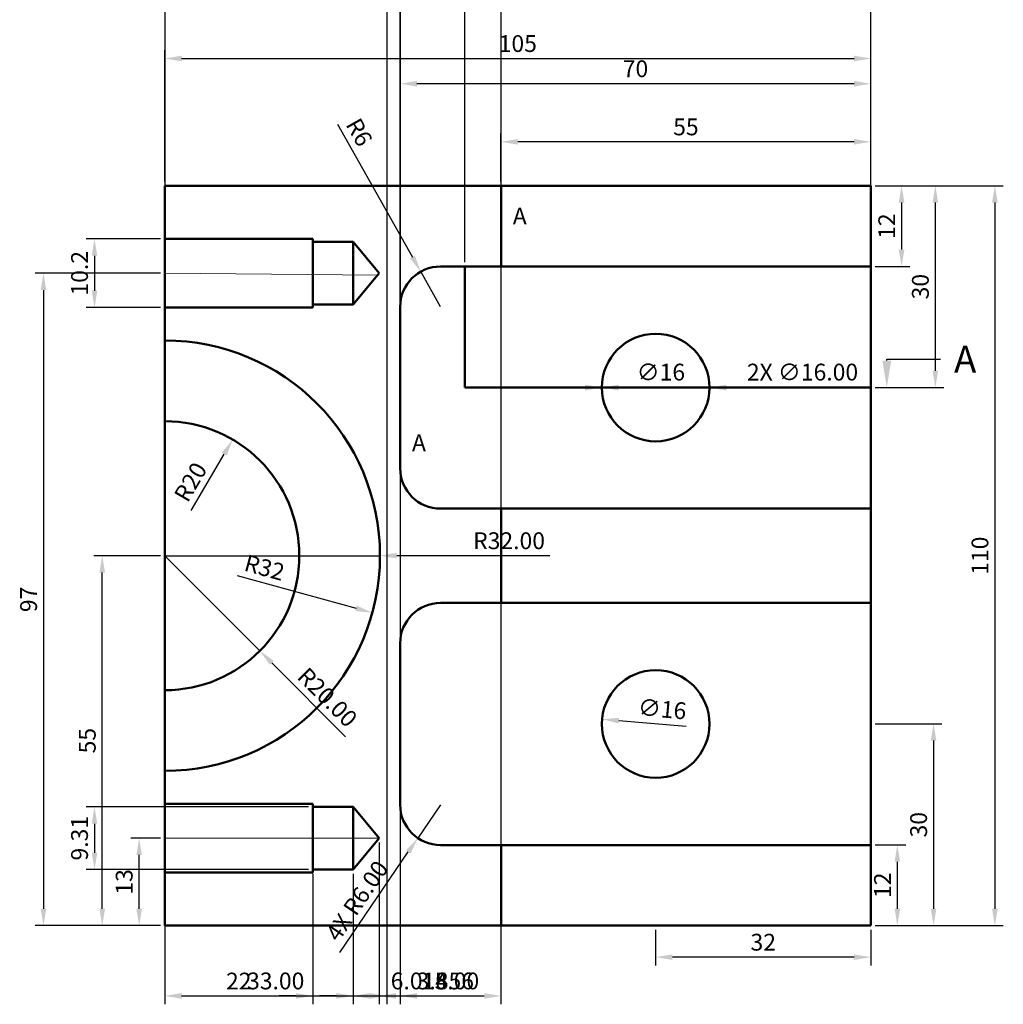
# Model space of a CAD drawing. Units: millimetres. Extents: x 2319 to 2465, y 1802 to 2026.
# Tile 1 of 2: x 2319 to 2465, y 1802 to 1949. Entities that reach past the tile are written whole.
import ezdxf
from ezdxf import colors
from ezdxf.entities.mleader import LeaderData, LeaderLine
from ezdxf.math import Vec2, Vec3

# ---------------------------------------------------------------- set-up
doc = ezdxf.new("R2010")
doc.units = ezdxf.units.MM
doc.linetypes.add('CENTER', pattern=[50.8, 31.75, -6.35, 6.35, -6.35])
for name, color, linetype, lineweight in [('M-CNTR', 1, 'CENTER', 18), ('M-DIMS', 2, 'Continuous', 25), ('M-OUTL', 7, 'Continuous', 50), ('M-TEXT', 3, 'Continuous', 25)]:
    doc.layers.add(name, color=color, linetype=linetype, lineweight=lineweight)
doc.styles.get("Standard").update_dxf_attribs({"font": 'arial.ttf'})
doc.dimstyles.new('ISO-25', dxfattribs={"dimtxt": 2.5, "dimasz": 2.5, "dimexe": 1.25, "dimexo": 0.625, "dimtad": 1, "dimtxsty": 'Standard', "dimcen": 2.5, "dimadec": 0, "dimazin": 0, "dimtfac": 1, "dimtmove": 0, "dimatfit": 3, "dimfxl": 1, "dimarcsym": 0})

# ---------------------------------------------------------------- blocks, each defined once
blk = doc.blocks.new('*D9')
at = {"layer": 'Defpoints', "color": 0, "transparency": 16777216}
for p in [(2378.57, 1911.38), (2381.51, 1906.15)]:
    blk.add_point(p, dxfattribs=at)
at = {"layer": 'M-DIMS', "color": 0, "lineweight": -2, "transparency": 16777216}
for p, q in [((2366.19, 1933.32), (2377.34, 1913.55)), ((2381.51, 1906.15), (2378.57, 1911.38))]:
    blk.add_line(p, q, dxfattribs=at)
at = {"layer": 'M-DIMS', "color": 0, "transparency": 16777216}
blk.add_solid([(2377.7, 1913.76), (2376.98, 1913.35), (2378.57, 1911.38)], dxfattribs=at)
at = {"layer": 'M-DIMS', "color": 0, "transparency": 16777216, "insert": (2369.14, 1931.95), "char_height": 2.5, "attachment_point": 5, "rotation": 299.424}
blk.add_mtext('R6', dxfattribs=at)
blk = doc.blocks.new('*D10')
at = {"layer": 'Defpoints', "color": 0, "transparency": 16777216}
for p in [(2350.61, 1886.41), (2340.51, 1869.15)]:
    blk.add_point(p, dxfattribs=at)
at = {"layer": 'M-DIMS', "color": 0, "lineweight": -2, "transparency": 16777216}
blk.add_line((2344.44, 1875.87), (2349.35, 1884.26), dxfattribs=at)
at = {"layer": 'M-DIMS', "color": 0, "transparency": 16777216}
blk.add_solid([(2348.99, 1884.47), (2349.71, 1884.05), (2350.61, 1886.41)], dxfattribs=at)
at = {"layer": 'M-DIMS', "color": 0, "transparency": 16777216, "insert": (2344.62, 1879.94), "char_height": 2.5, "attachment_point": 5, "rotation": 59.6796}
blk.add_mtext('R20', dxfattribs=at)
blk = doc.blocks.new('*D11')
at = {"layer": 'Defpoints', "color": 0, "transparency": 16777216}
for p in [(2340.51, 1869.15), (2371.37, 1860.67)]:
    blk.add_point(p, dxfattribs=at)
at = {"layer": 'M-DIMS', "color": 0, "lineweight": -2, "transparency": 16777216}
blk.add_line((2351.29, 1866.19), (2368.96, 1861.33), dxfattribs=at)
at = {"layer": 'M-DIMS', "color": 0, "transparency": 16777216}
blk.add_solid([(2369.07, 1861.73), (2368.85, 1860.93), (2371.37, 1860.67)], dxfattribs=at)
at = {"layer": 'M-DIMS', "color": 0, "transparency": 16777216, "insert": (2355.26, 1867.07), "char_height": 2.5, "attachment_point": 5, "rotation": 344.6335}
blk.add_mtext('R32', dxfattribs=at)
blk = doc.blocks.new('*D12')
at = {"layer": 'Defpoints', "color": 0, "transparency": 16777216}
for p in [(2405.51, 1894.15), (2421.51, 1894.15)]:
    blk.add_point(p, dxfattribs=at)
at = {"layer": 'M-DIMS', "color": 0, "lineweight": -2, "transparency": 16777216}
blk.add_line((2418.06, 1894.15), (2408.01, 1894.15), dxfattribs=at)
at = {"layer": 'M-DIMS', "color": 0, "transparency": 16777216}
blk.add_solid([(2408.01, 1894.57), (2408.01, 1893.73), (2405.51, 1894.15)], dxfattribs=at)
at = {"layer": 'M-DIMS', "color": 0, "transparency": 16777216, "insert": (2414.29, 1896.12), "char_height": 2.5, "attachment_point": 5}
blk.add_mtext('∅16', dxfattribs=at)
blk = doc.blocks.new('*D13')
at = {"layer": 'Defpoints', "color": 0, "transparency": 16777216}
for p in [(2405.55, 1844.84), (2421.48, 1843.42)]:
    blk.add_point(p, dxfattribs=at)
at = {"layer": 'M-DIMS', "color": 0, "lineweight": -2, "transparency": 16777216}
blk.add_line((2418.05, 1843.73), (2408.04, 1844.62), dxfattribs=at)
at = {"layer": 'M-DIMS', "color": 0, "transparency": 16777216}
blk.add_solid([(2408.07, 1845.04), (2408, 1844.21), (2405.55, 1844.84)], dxfattribs=at)
at = {"layer": 'M-DIMS', "color": 0, "transparency": 16777216, "insert": (2414.46, 1846.03), "char_height": 2.5, "attachment_point": 5, "rotation": 354.9079}
blk.add_mtext('∅16', dxfattribs=at)
blk = doc.blocks.new('*D14')
at = {"layer": 'Defpoints', "color": 0, "transparency": 16777216}
for p in [(2445.51, 1943.07), (2340.51, 1924.15), (2445.51, 1924.15)]:
    blk.add_point(p, dxfattribs=at)
at = {"layer": 'M-DIMS', "color": 0, "lineweight": -2, "transparency": 16777216}
for p, q in [((2340.51, 1924.77), (2340.51, 1944.32)), ((2445.51, 1924.77), (2445.51, 1944.32)), ((2343.01, 1943.07), (2443.01, 1943.07))]:
    blk.add_line(p, q, dxfattribs=at)
at = {"layer": 'M-DIMS', "color": 0, "transparency": 16777216}
for points in [[(2343.01, 1943.49), (2343.01, 1942.65), (2340.51, 1943.07)], [(2443.01, 1943.49), (2443.01, 1942.65), (2445.51, 1943.07)]]:
    blk.add_solid(points, dxfattribs=at)
at = {"layer": 'M-DIMS', "color": 0, "transparency": 16777216, "insert": (2393.01, 1944.97), "char_height": 2.5, "attachment_point": 5}
blk.add_mtext('105', dxfattribs=at)
blk = doc.blocks.new('*D15')
at = {"layer": 'Defpoints', "color": 0, "transparency": 16777216}
for p in [(2375.51, 1939.32), (2375.51, 1924.15), (2445.51, 1924.15)]:
    blk.add_point(p, dxfattribs=at)
at = {"layer": 'M-DIMS', "color": 0, "lineweight": -2, "transparency": 16777216}
for p, q in [((2375.51, 1924.77), (2375.51, 1940.57)), ((2445.51, 1924.77), (2445.51, 1940.57)), ((2443.01, 1939.32), (2378.01, 1939.32))]:
    blk.add_line(p, q, dxfattribs=at)
at = {"layer": 'M-DIMS', "color": 0, "transparency": 16777216}
for points in [[(2378.01, 1939.74), (2378.01, 1938.9), (2375.51, 1939.32)], [(2443.01, 1939.74), (2443.01, 1938.9), (2445.51, 1939.32)]]:
    blk.add_solid(points, dxfattribs=at)
at = {"layer": 'M-DIMS', "color": 0, "transparency": 16777216, "insert": (2410.51, 1941.22), "char_height": 2.5, "attachment_point": 5}
blk.add_mtext('70', dxfattribs=at)
blk = doc.blocks.new('*D16')
at = {"layer": 'Defpoints', "color": 0, "transparency": 16777216}
for p in [(2390.51, 1930.68), (2390.51, 1924.15), (2445.51, 1924.15)]:
    blk.add_point(p, dxfattribs=at)
at = {"layer": 'M-DIMS', "color": 0, "lineweight": -2, "transparency": 16777216}
for p, q in [((2390.51, 1924.77), (2390.51, 1931.93)), ((2445.51, 1924.77), (2445.51, 1931.93)), ((2443.01, 1930.68), (2393.01, 1930.68))]:
    blk.add_line(p, q, dxfattribs=at)
at = {"layer": 'M-DIMS', "color": 0, "transparency": 16777216}
for points in [[(2393.01, 1931.1), (2393.01, 1930.27), (2390.51, 1930.68)], [(2443.01, 1931.1), (2443.01, 1930.27), (2445.51, 1930.68)]]:
    blk.add_solid(points, dxfattribs=at)
at = {"layer": 'M-DIMS', "color": 0, "transparency": 16777216, "insert": (2418.01, 1932.58), "char_height": 2.5, "attachment_point": 5}
blk.add_mtext('55', dxfattribs=at)
blk = doc.blocks.new('*D17')
at = {"layer": 'Defpoints', "color": 0, "transparency": 16777216}
for p in [(2445.51, 1924.15), (2445.51, 1912.15), (2450.08, 1912.15)]:
    blk.add_point(p, dxfattribs=at)
at = {"layer": 'M-DIMS', "color": 0, "lineweight": -2, "transparency": 16777216}
for p, q in [((2446.14, 1924.15), (2451.33, 1924.15)), ((2450.08, 1921.65), (2450.08, 1914.65)), ((2446.14, 1912.15), (2451.33, 1912.15))]:
    blk.add_line(p, q, dxfattribs=at)
at = {"layer": 'M-DIMS', "color": 0, "transparency": 16777216}
for points in [[(2449.66, 1921.65), (2450.5, 1921.65), (2450.08, 1924.15)], [(2449.66, 1914.65), (2450.5, 1914.65), (2450.08, 1912.15)]]:
    blk.add_solid(points, dxfattribs=at)
at = {"layer": 'M-DIMS', "color": 0, "transparency": 16777216, "insert": (2448.2, 1918.15), "char_height": 2.5, "attachment_point": 5, "rotation": 90}
blk.add_mtext('12', dxfattribs=at)
blk = doc.blocks.new('*D18')
at = {"layer": 'Defpoints', "color": 0, "transparency": 16777216}
for p in [(2445.51, 1924.15), (2445.51, 1894.15), (2455.1, 1894.15)]:
    blk.add_point(p, dxfattribs=at)
at = {"layer": 'M-DIMS', "color": 0, "lineweight": -2, "transparency": 16777216}
for p, q in [((2446.14, 1924.15), (2456.35, 1924.15)), ((2455.1, 1921.65), (2455.1, 1896.65)), ((2446.14, 1894.15), (2456.35, 1894.15))]:
    blk.add_line(p, q, dxfattribs=at)
at = {"layer": 'M-DIMS', "color": 0, "transparency": 16777216}
for points in [[(2454.69, 1921.65), (2455.52, 1921.65), (2455.1, 1924.15)], [(2454.69, 1896.65), (2455.52, 1896.65), (2455.1, 1894.15)]]:
    blk.add_solid(points, dxfattribs=at)
at = {"layer": 'M-DIMS', "color": 0, "transparency": 16777216, "insert": (2453.2, 1909.15), "char_height": 2.5, "attachment_point": 5, "rotation": 90}
blk.add_mtext('30', dxfattribs=at)
blk = doc.blocks.new('*D19')
at = {"layer": 'Defpoints', "color": 0, "transparency": 16777216}
for p in [(2445.51, 1924.15), (2445.51, 1814.15), (2463.96, 1814.15)]:
    blk.add_point(p, dxfattribs=at)
at = {"layer": 'M-DIMS', "color": 0, "lineweight": -2, "transparency": 16777216}
for p, q in [((2446.14, 1924.15), (2465.21, 1924.15)), ((2463.96, 1921.65), (2463.96, 1816.65)), ((2446.14, 1814.15), (2465.21, 1814.15))]:
    blk.add_line(p, q, dxfattribs=at)
at = {"layer": 'M-DIMS', "color": 0, "transparency": 16777216}
for points in [[(2463.54, 1921.65), (2464.38, 1921.65), (2463.96, 1924.15)], [(2463.54, 1816.65), (2464.38, 1816.65), (2463.96, 1814.15)]]:
    blk.add_solid(points, dxfattribs=at)
at = {"layer": 'M-DIMS', "color": 0, "transparency": 16777216, "insert": (2462.06, 1869.15), "char_height": 2.5, "attachment_point": 5, "rotation": 90}
blk.add_mtext('110', dxfattribs=at)
blk = doc.blocks.new('*D20')
at = {"layer": 'Defpoints', "color": 0, "transparency": 16777216}
for p in [(2445.51, 1826.15), (2449.45, 1826.15), (2445.51, 1814.15)]:
    blk.add_point(p, dxfattribs=at)
at = {"layer": 'M-DIMS', "color": 0, "lineweight": -2, "transparency": 16777216}
for p, q in [((2446.14, 1826.15), (2450.7, 1826.15)), ((2449.45, 1816.65), (2449.45, 1823.65)), ((2446.14, 1814.15), (2450.7, 1814.15))]:
    blk.add_line(p, q, dxfattribs=at)
at = {"layer": 'M-DIMS', "color": 0, "transparency": 16777216}
for points in [[(2449.04, 1823.65), (2449.87, 1823.65), (2449.45, 1826.15)], [(2449.04, 1816.65), (2449.87, 1816.65), (2449.45, 1814.15)]]:
    blk.add_solid(points, dxfattribs=at)
at = {"layer": 'M-DIMS', "color": 0, "transparency": 16777216, "insert": (2447.57, 1820.15), "char_height": 2.5, "attachment_point": 5, "rotation": 90}
blk.add_mtext('12', dxfattribs=at)
blk = doc.blocks.new('*D21')
at = {"layer": 'Defpoints', "color": 0, "transparency": 16777216}
for p in [(2445.51, 1844.15), (2445.51, 1814.15), (2454.84, 1814.15)]:
    blk.add_point(p, dxfattribs=at)
at = {"layer": 'M-DIMS', "color": 0, "lineweight": -2, "transparency": 16777216}
for p, q in [((2446.14, 1844.15), (2456.09, 1844.15)), ((2454.84, 1841.65), (2454.84, 1816.65)), ((2446.14, 1814.15), (2456.09, 1814.15))]:
    blk.add_line(p, q, dxfattribs=at)
at = {"layer": 'M-DIMS', "color": 0, "transparency": 16777216}
for points in [[(2454.42, 1841.65), (2455.25, 1841.65), (2454.84, 1844.15)], [(2454.42, 1816.65), (2455.25, 1816.65), (2454.84, 1814.15)]]:
    blk.add_solid(points, dxfattribs=at)
at = {"layer": 'M-DIMS', "color": 0, "transparency": 16777216, "insert": (2452.94, 1829.15), "char_height": 2.5, "attachment_point": 5, "rotation": 90}
blk.add_mtext('30', dxfattribs=at)
blk = doc.blocks.new('*D22')
at = {"layer": 'Defpoints', "color": 0, "transparency": 16777216}
for p in [(2413.51, 1814.15), (2445.51, 1814.15), (2413.51, 1809.46)]:
    blk.add_point(p, dxfattribs=at)
at = {"layer": 'M-DIMS', "color": 0, "lineweight": -2, "transparency": 16777216}
for p, q in [((2413.51, 1813.52), (2413.51, 1808.21)), ((2445.51, 1813.52), (2445.51, 1808.21)), ((2443.01, 1809.46), (2416.01, 1809.46))]:
    blk.add_line(p, q, dxfattribs=at)
at = {"layer": 'M-DIMS', "color": 0, "transparency": 16777216}
for points in [[(2416.01, 1809.87), (2416.01, 1809.04), (2413.51, 1809.46)], [(2443.01, 1809.87), (2443.01, 1809.04), (2445.51, 1809.46)]]:
    blk.add_solid(points, dxfattribs=at)
at = {"layer": 'M-DIMS', "color": 0, "transparency": 16777216, "insert": (2429.51, 1811.36), "char_height": 2.5, "attachment_point": 5}
blk.add_mtext('32', dxfattribs=at)
blk = doc.blocks.new('*D23')
at = {"layer": 'Defpoints', "color": 0, "transparency": 16777216}
for p in [(2336.7, 1827.15), (2340.51, 1827.15), (2340.51, 1814.15)]:
    blk.add_point(p, dxfattribs=at)
at = {"layer": 'M-DIMS', "color": 0, "lineweight": -2, "transparency": 16777216}
for p, q in [((2339.89, 1827.15), (2335.45, 1827.15)), ((2336.7, 1816.65), (2336.7, 1824.65)), ((2339.89, 1814.15), (2335.45, 1814.15))]:
    blk.add_line(p, q, dxfattribs=at)
at = {"layer": 'M-DIMS', "color": 0, "transparency": 16777216}
for points in [[(2336.29, 1824.65), (2337.12, 1824.65), (2336.7, 1827.15)], [(2336.29, 1816.65), (2337.12, 1816.65), (2336.7, 1814.15)]]:
    blk.add_solid(points, dxfattribs=at)
at = {"layer": 'M-DIMS', "color": 0, "transparency": 16777216, "insert": (2334.8, 1820.65), "char_height": 2.5, "attachment_point": 5, "rotation": 90}
blk.add_mtext('13', dxfattribs=at)
blk = doc.blocks.new('*D24')
at = {"layer": 'Defpoints', "color": 0, "transparency": 16777216}
for p in [(2331.21, 1869.15), (2340.51, 1869.15), (2340.51, 1814.15)]:
    blk.add_point(p, dxfattribs=at)
at = {"layer": 'M-DIMS', "color": 0, "lineweight": -2, "transparency": 16777216}
for p, q in [((2339.89, 1869.15), (2329.96, 1869.15)), ((2331.21, 1816.65), (2331.21, 1866.65)), ((2339.89, 1814.15), (2329.96, 1814.15))]:
    blk.add_line(p, q, dxfattribs=at)
at = {"layer": 'M-DIMS', "color": 0, "transparency": 16777216}
for points in [[(2330.79, 1866.65), (2331.63, 1866.65), (2331.21, 1869.15)], [(2330.79, 1816.65), (2331.63, 1816.65), (2331.21, 1814.15)]]:
    blk.add_solid(points, dxfattribs=at)
at = {"layer": 'M-DIMS', "color": 0, "transparency": 16777216, "insert": (2329.31, 1841.65), "char_height": 2.5, "attachment_point": 5, "rotation": 90}
blk.add_mtext('55', dxfattribs=at)
blk = doc.blocks.new('*D25')
at = {"layer": 'Defpoints', "color": 0, "transparency": 16777216}
for p in [(2340.51, 1911.15), (2322.48, 1814.15), (2340.51, 1814.15)]:
    blk.add_point(p, dxfattribs=at)
at = {"layer": 'M-DIMS', "color": 0, "lineweight": -2, "transparency": 16777216}
for p, q in [((2339.89, 1911.15), (2321.23, 1911.15)), ((2322.48, 1908.65), (2322.48, 1816.65)), ((2339.89, 1814.15), (2321.23, 1814.15))]:
    blk.add_line(p, q, dxfattribs=at)
at = {"layer": 'M-DIMS', "color": 0, "transparency": 16777216}
for points in [[(2322.06, 1908.65), (2322.89, 1908.65), (2322.48, 1911.15)], [(2322.06, 1816.65), (2322.89, 1816.65), (2322.48, 1814.15)]]:
    blk.add_solid(points, dxfattribs=at)
at = {"layer": 'M-DIMS', "color": 0, "transparency": 16777216, "insert": (2320.58, 1862.65), "char_height": 2.5, "attachment_point": 5, "rotation": 90}
blk.add_mtext('97', dxfattribs=at)
blk = doc.blocks.new('TAPPED-HOLE')
for p, q in [((0, 10.21), (22, 10.21)), ((22, 10.21), (22, 0.01)), ((22, 10.2), (22, 0)), ((22, 9.78), (28.01, 9.78)), ((22, 5.1), (22, 9.76)), ((28.01, 9.78), (28.01, 0.45)), ((31.87, 5.11), (28.01, 9.78)), ((28.01, 0.45), (31.87, 5.11)), ((22, 0.01), (0, 0.01)), ((22, 0.45), (28.01, 0.45))]:
    blk.add_line(p, q)
blk = doc.blocks.new('*D27')
at = {"layer": 'Defpoints', "color": 0, "transparency": 16777216}
for p in [(2340.51, 1822.05), (2362.51, 1822.04), (2362.51, 1803.7)]:
    blk.add_point(p, dxfattribs=at)
at = {"layer": 'M-DIMS', "color": 0, "lineweight": -2, "transparency": 16777216}
for p, q in [((2340.51, 1821.42), (2340.51, 1802.45)), ((2362.51, 1821.41), (2362.51, 1802.45)), ((2343.01, 1803.7), (2360.01, 1803.7))]:
    blk.add_line(p, q, dxfattribs=at)
at = {"layer": 'M-DIMS', "color": 0, "transparency": 16777216}
for points in [[(2343.01, 1804.12), (2343.01, 1803.28), (2340.51, 1803.7)], [(2360.01, 1804.12), (2360.01, 1803.28), (2362.51, 1803.7)]]:
    blk.add_solid(points, dxfattribs=at)
at = {"layer": 'M-DIMS', "color": 0, "transparency": 16777216, "insert": (2351.51, 1805.58), "char_height": 2.5, "attachment_point": 5}
blk.add_mtext('22', dxfattribs=at)
blk = doc.blocks.new('*D28')
at = {"layer": 'Defpoints', "color": 0, "transparency": 16777216}
for p in [(2362.51, 1822.49), (2368.53, 1822.49), (2368.53, 1803.7)]:
    blk.add_point(p, dxfattribs=at)
at = {"layer": 'M-DIMS', "color": 0, "lineweight": -2, "transparency": 16777216}
for p, q in [((2362.51, 1821.86), (2362.51, 1802.45)), ((2368.53, 1821.86), (2368.53, 1802.45)), ((2360.01, 1803.7), (2357.51, 1803.7)), ((2362.51, 1803.7), (2368.53, 1803.7)), ((2371.03, 1803.7), (2383.22, 1803.7))]:
    blk.add_line(p, q, dxfattribs=at)
at = {"layer": 'M-DIMS', "color": 0, "transparency": 16777216}
for points in [[(2360.01, 1804.12), (2360.01, 1803.28), (2362.51, 1803.7)], [(2371.03, 1804.12), (2371.03, 1803.28), (2368.53, 1803.7)]]:
    blk.add_solid(points, dxfattribs=at)
at = {"layer": 'M-DIMS', "color": 0, "transparency": 16777216, "insert": (2378.37, 1805.6), "char_height": 2.5, "attachment_point": 5}
blk.add_mtext('6.014', dxfattribs=at)
blk = doc.blocks.new('*D29')
at = {"layer": 'Defpoints', "color": 0, "transparency": 16777216}
for p in [(2372.38, 1827.15), (2368.53, 1822.49), (2372.38, 1803.7)]:
    blk.add_point(p, dxfattribs=at)
at = {"layer": 'M-DIMS', "color": 0, "lineweight": -2, "transparency": 16777216}
for p, q in [((2372.38, 1826.52), (2372.38, 1802.45)), ((2368.53, 1821.86), (2368.53, 1802.45)), ((2366.03, 1803.7), (2363.53, 1803.7)), ((2368.53, 1803.7), (2372.38, 1803.7)), ((2374.88, 1803.7), (2387.07, 1803.7))]:
    blk.add_line(p, q, dxfattribs=at)
at = {"layer": 'M-DIMS', "color": 0, "transparency": 16777216}
for points in [[(2366.03, 1804.12), (2366.03, 1803.28), (2368.53, 1803.7)], [(2374.88, 1804.12), (2374.88, 1803.28), (2372.38, 1803.7)]]:
    blk.add_solid(points, dxfattribs=at)
at = {"layer": 'M-DIMS', "color": 0, "transparency": 16777216, "insert": (2382.23, 1805.6), "char_height": 2.5, "attachment_point": 5}
blk.add_mtext('3.856', dxfattribs=at)
blk = doc.blocks.new('*D30')
at = {"layer": 'Defpoints', "color": 0, "transparency": 16777216}
for p in [(2340.51, 1916.24), (2330.06, 1906.04), (2340.51, 1906.04)]:
    blk.add_point(p, dxfattribs=at)
at = {"layer": 'M-DIMS', "color": 0, "lineweight": -2, "transparency": 16777216}
for p, q in [((2339.89, 1916.24), (2328.81, 1916.24)), ((2330.06, 1913.74), (2330.06, 1908.54)), ((2339.89, 1906.04), (2328.81, 1906.04))]:
    blk.add_line(p, q, dxfattribs=at)
at = {"layer": 'M-DIMS', "color": 0, "transparency": 16777216}
for points in [[(2329.65, 1913.74), (2330.48, 1913.74), (2330.06, 1916.24)], [(2329.65, 1908.54), (2330.48, 1908.54), (2330.06, 1906.04)]]:
    blk.add_solid(points, dxfattribs=at)
at = {"layer": 'M-DIMS', "color": 0, "transparency": 16777216, "insert": (2328.16, 1911.14), "char_height": 2.5, "attachment_point": 5, "rotation": 90}
blk.add_mtext('10.2', dxfattribs=at)
blk = doc.blocks.new('*D31')
at = {"layer": 'Defpoints', "color": 0, "transparency": 16777216}
for p in [(2362.51, 1831.8), (2330.06, 1822.49), (2362.51, 1822.49)]:
    blk.add_point(p, dxfattribs=at)
at = {"layer": 'M-DIMS', "color": 0, "lineweight": -2, "transparency": 16777216}
for p, q in [((2361.89, 1831.8), (2328.81, 1831.8)), ((2330.06, 1829.3), (2330.06, 1824.99)), ((2361.89, 1822.49), (2328.81, 1822.49))]:
    blk.add_line(p, q, dxfattribs=at)
at = {"layer": 'M-DIMS', "color": 0, "transparency": 16777216}
for points in [[(2329.65, 1829.3), (2330.48, 1829.3), (2330.06, 1831.8)], [(2329.65, 1824.99), (2330.48, 1824.99), (2330.06, 1822.49)]]:
    blk.add_solid(points, dxfattribs=at)
at = {"layer": 'M-DIMS', "color": 0, "transparency": 16777216, "insert": (2328.16, 1827.14), "char_height": 2.5, "attachment_point": 5, "rotation": 90}
blk.add_mtext('9.31', dxfattribs=at)
blk = doc.blocks.new('*D32')
at = {"layer": 'Defpoints', "color": 0, "transparency": 16777216}
for p in [(2445.51, 2022.1), (2385.13, 1912.15), (2445.51, 1912.15)]:
    blk.add_point(p, dxfattribs=at)
at = {"layer": 'M-DIMS', "color": 0, "lineweight": -2, "transparency": 16777216}
for p, q in [((2385.13, 1912.77), (2385.13, 2023.35)), ((2445.51, 1912.77), (2445.51, 2023.35)), ((2387.63, 2022.1), (2443.01, 2022.1))]:
    blk.add_line(p, q, dxfattribs=at)
at = {"layer": 'M-DIMS', "color": 0, "transparency": 16777216}
for points in [[(2387.63, 2022.52), (2387.63, 2021.68), (2385.13, 2022.1)], [(2443.01, 2022.52), (2443.01, 2021.68), (2445.51, 2022.1)]]:
    blk.add_solid(points, dxfattribs=at)
at = {"layer": 'M-DIMS', "color": 0, "transparency": 16777216, "insert": (2415.32, 2024), "char_height": 2.5, "attachment_point": 5}
blk.add_mtext('60.38', dxfattribs=at)
blk = doc.blocks.new('*D36')
at = {"layer": 'Defpoints', "color": 0, "transparency": 16777216}
for p in [(2340.51, 1961.65), (2373.51, 1961.65), (2373.51, 1803.7)]:
    blk.add_point(p, dxfattribs=at)
at = {"layer": 'M-DIMS', "color": 0, "lineweight": -2, "transparency": 16777216}
for p, q in [((2340.51, 1961.03), (2340.51, 1802.45)), ((2373.51, 1961.03), (2373.51, 1802.45)), ((2343.01, 1803.7), (2371.01, 1803.7))]:
    blk.add_line(p, q, dxfattribs=at)
at = {"layer": 'M-DIMS', "color": 0, "transparency": 16777216}
for points in [[(2343.01, 1804.12), (2343.01, 1803.28), (2340.51, 1803.7)], [(2371.01, 1804.12), (2371.01, 1803.28), (2373.51, 1803.7)]]:
    blk.add_solid(points, dxfattribs=at)
at = {"layer": 'M-DIMS', "color": 0, "transparency": 16777216, "insert": (2357.01, 1805.6), "char_height": 2.5, "attachment_point": 5}
blk.add_mtext('33.00', dxfattribs=at)
blk = doc.blocks.new('*D37')
at = {"layer": 'Defpoints', "color": 0, "transparency": 16777216}
for p in [(2375.51, 1966.65), (2390.51, 1966.65), (2390.51, 1803.7)]:
    blk.add_point(p, dxfattribs=at)
at = {"layer": 'M-DIMS', "color": 0, "lineweight": -2, "transparency": 16777216}
for p, q in [((2375.51, 1966.03), (2375.51, 1802.45)), ((2390.51, 1966.03), (2390.51, 1802.45)), ((2378.01, 1803.7), (2388.01, 1803.7))]:
    blk.add_line(p, q, dxfattribs=at)
at = {"layer": 'M-DIMS', "color": 0, "transparency": 16777216}
for points in [[(2378.01, 1804.12), (2378.01, 1803.28), (2375.51, 1803.7)], [(2388.01, 1804.12), (2388.01, 1803.28), (2390.51, 1803.7)]]:
    blk.add_solid(points, dxfattribs=at)
at = {"layer": 'M-DIMS', "color": 0, "transparency": 16777216, "insert": (2383.01, 1805.6), "char_height": 2.5, "attachment_point": 5}
blk.add_mtext('15.00', dxfattribs=at)
blk = doc.blocks.new('*D38')
at = {"layer": 'Defpoints', "color": 0, "transparency": 16777216}
for p in [(2385.13, 2022.1), (2385.13, 1912.15), (2375.51, 1906.15)]:
    blk.add_point(p, dxfattribs=at)
at = {"layer": 'M-DIMS', "color": 0, "lineweight": -2, "transparency": 16777216}
for p, q in [((2375.51, 1906.77), (2375.51, 2023.35)), ((2385.13, 1912.77), (2385.13, 2023.35)), ((2378.01, 2022.1), (2382.63, 2022.1)), ((2385.13, 2022.1), (2397.32, 2022.1))]:
    blk.add_line(p, q, dxfattribs=at)
at = {"layer": 'M-DIMS', "color": 0, "transparency": 16777216}
for points in [[(2378.01, 2022.52), (2378.01, 2021.68), (2375.51, 2022.1)], [(2382.63, 2022.52), (2382.63, 2021.68), (2385.13, 2022.1)]]:
    blk.add_solid(points, dxfattribs=at)
at = {"layer": 'M-DIMS', "color": 0, "transparency": 16777216, "insert": (2392.47, 2024), "char_height": 2.5, "attachment_point": 5}
blk.add_mtext('9.617', dxfattribs=at)
blk = doc.blocks.new('*D39')
at = {"layer": 'Defpoints', "color": 0, "transparency": 16777216}
for p in [(2340.51, 1869.15), (2372.51, 1869.15)]:
    blk.add_point(p, dxfattribs=at)
at = {"layer": 'M-DIMS', "color": 0, "lineweight": -2, "transparency": 16777216}
for p, q in [((2340.51, 1869.15), (2372.51, 1869.15)), ((2397.75, 1869.15), (2375.01, 1869.15))]:
    blk.add_line(p, q, dxfattribs=at)
at = {"layer": 'M-DIMS', "color": 0, "transparency": 16777216}
blk.add_solid([(2375.01, 1869.57), (2375.01, 1868.73), (2372.51, 1869.15)], dxfattribs=at)
at = {"layer": 'M-DIMS', "color": 0, "transparency": 16777216, "insert": (2391.71, 1871.05), "char_height": 2.5, "attachment_point": 5, "rotation": 0.0005}
blk.add_mtext('R32.00', dxfattribs=at)
blk = doc.blocks.new('*D40')
at = {"layer": 'Defpoints', "color": 0, "transparency": 16777216}
for p in [(2340.51, 1869.15), (2354.65, 1855)]:
    blk.add_point(p, dxfattribs=at)
at = {"layer": 'M-DIMS', "color": 0, "lineweight": -2, "transparency": 16777216}
for p, q in [((2340.51, 1869.15), (2354.65, 1855)), ((2367.4, 1842.24), (2356.42, 1853.23))]:
    blk.add_line(p, q, dxfattribs=at)
at = {"layer": 'M-DIMS', "color": 0, "transparency": 16777216}
blk.add_solid([(2356.71, 1853.53), (2356.12, 1852.94), (2354.65, 1855)], dxfattribs=at)
at = {"layer": 'M-DIMS', "color": 0, "transparency": 16777216, "insert": (2364.48, 1847.86), "char_height": 2.5, "attachment_point": 5, "rotation": 314.9722}
blk.add_mtext('R20.00', dxfattribs=at)
blk = doc.blocks.new('*D41')
at = {"layer": 'Defpoints', "color": 0, "transparency": 16777216}
for p in [(2405.51, 1894.15), (2421.51, 1894.15)]:
    blk.add_point(p, dxfattribs=at)
at = {"layer": 'M-DIMS', "color": 0, "lineweight": -2, "transparency": 16777216}
for p, q in [((2403.01, 1894.15), (2400.51, 1894.15)), ((2405.51, 1894.15), (2421.51, 1894.15)), ((2444.19, 1894.15), (2424.01, 1894.15))]:
    blk.add_line(p, q, dxfattribs=at)
at = {"layer": 'M-DIMS', "color": 0, "transparency": 16777216}
for points in [[(2403.01, 1894.57), (2403.01, 1893.73), (2405.51, 1894.15)], [(2424.01, 1894.57), (2424.01, 1893.73), (2421.51, 1894.15)]]:
    blk.add_solid(points, dxfattribs=at)
at = {"layer": 'M-DIMS', "color": 0, "transparency": 16777216, "insert": (2435.35, 1896.12), "char_height": 2.5, "attachment_point": 5, "rotation": 0.0022}
blk.add_mtext('2X ∅16.00', dxfattribs=at)
blk = doc.blocks.new('*D42')
at = {"layer": 'Defpoints', "color": 0, "transparency": 16777216}
for p in [(2381.51, 1832.13), (2378.14, 1827.17)]:
    blk.add_point(p, dxfattribs=at)
at = {"layer": 'M-DIMS', "color": 0, "lineweight": -2, "transparency": 16777216}
for p, q in [((2381.51, 1832.13), (2378.14, 1827.17)), ((2366.54, 1810.15), (2376.73, 1825.11))]:
    blk.add_line(p, q, dxfattribs=at)
at = {"layer": 'M-DIMS', "color": 0, "transparency": 16777216}
blk.add_solid([(2376.39, 1825.34), (2377.07, 1824.87), (2378.14, 1827.17)], dxfattribs=at)
at = {"layer": 'M-DIMS', "color": 0, "transparency": 16777216, "insert": (2369.36, 1817.66), "char_height": 2.5, "attachment_point": 5, "rotation": 55.7461}
blk.add_mtext('4X R6.00', dxfattribs=at)

msp = doc.modelspace()

# ---------------------------------------------------------------- linework, layer by layer
at = {"layer": 'M-CNTR'}
for p, q in [((2340.514, 1911.1497), (2377.7092, 1910.7891)), ((2340.514, 1827.1497), (2373.5308, 1827.1497))]:
    msp.add_line(p, q, dxfattribs=at)
at = {"layer": 'M-OUTL'}
for p, q in [((2346.514, 1924.1497), (2340.514, 1924.1497)), ((2340.514, 1924.1497), (2340.514, 1918.1497)), ((2346.514, 1924.1497), (2445.514, 1924.1497)), ((2390.514, 1924.1497), (2390.514, 1912.1497)), ((2445.514, 1924.1497), (2445.514, 1814.1497)), ((2445.514, 1924.1497), (2445.514, 1912.1497)), ((2445.514, 1924.1497), (2445.514, 1894.1497)), ((2340.514, 1889.1497), (2340.514, 1918.1497)), ((2445.514, 1912.1497), (2381.514, 1912.1497)), ((2385.1309, 1894.1497), (2385.1309, 1912.1497)), ((2340.514, 1814.1497), (2340.514, 1911.1497)), ((2375.514, 1906.1497), (2375.514, 1882.1497)), ((2445.514, 1894.1497), (2385.1309, 1894.1497)), ((2381.514, 1876.1497), (2445.514, 1876.1497)), ((2390.514, 1876.1497), (2390.514, 1862.1323)), ((2445.514, 1862.1323), (2381.514, 1862.1323)), ((2375.514, 1856.1323), (2375.514, 1832.1323)), ((2340.514, 1814.1497), (2340.514, 1849.1497)), ((2340.514, 1814.1497), (2340.514, 1849.1497)), ((2445.514, 1814.1497), (2445.514, 1846.1497)), ((2445.514, 1846.1497), (2445.514, 1844.1497)), ((2340.514, 1814.1497), (2340.514, 1827.1497)), ((2381.514, 1826.1323), (2445.514, 1826.1323)), ((2390.514, 1826.1323), (2390.514, 1814.1497)), ((2445.514, 1814.1497), (2340.514, 1814.1497))]:
    msp.add_line(p, q, dxfattribs=at)
for centre in [(2413.514, 1894.1497), (2413.514, 1844.1323)]:
    msp.add_circle(centre, 8, dxfattribs=at)
for centre, radius, start, end in [((2381.514, 1906.1497), 6, 90, 180), ((2340.514, 1869.1497), 32, 270, 90), ((2340.514, 1869.1497), 20, 270, 90), ((2381.514, 1882.1497), 6, 180, 270), ((2381.514, 1856.1323), 6, 90, 180), ((2381.514, 1832.1323), 6, 180, 270)]:
    msp.add_arc(centre, radius, start, end, dxfattribs=at)

# ---------------------------------------------------------------- block references
for p in [(2340.514, 1906.029), (2340.514, 1822.0371)]:
    msp.add_blockref('TAPPED-HOLE', p, dxfattribs=at)

# ---------------------------------------------------------------- texts
at = {"layer": 'M-TEXT', "char_height": 2.5, "attachment_point": 1}
for width, insert in [(7.236938, (2392.264, 1920.8934)), (8.576691, (2377.2752, 1887.1867))]:
    msp.add_mtext_dynamic_manual_height_columns('A', width=width, gutter_width=12.5, heights=[0], dxfattribs=dict(at, insert=insert))

# ---------------------------------------------------------------- dimensions: what is measured, and where the dimension line sits
at = {"layer": 'M-DIMS'}
for base, p1, p2, override, picture, middle in [((2385.1309, 2022.1002), (2375.514, 1906.1497), (2385.1309, 1912.1497), {"dimdec": 3, "dimlfac": 1, "dimrnd": 0, "dimzin": 0, "dimdsep": 46, "dimlunit": 2}, '*D38', (2392.474, 2024.0017)), ((2445.514, 2022.1002), (2385.1309, 1912.1497), (2445.514, 1912.1497), {"dimdec": 2, "dimlfac": 1, "dimrnd": 0, "dimzin": 0, "dimdsep": 46, "dimlunit": 2}, '*D32', (2415.3224, 2024.0025)), ((2390.514, 1803.6997), (2375.514, 1966.6502), (2390.514, 1966.6502), {"dimdec": 2, "dimlfac": 1, "dimrnd": 0, "dimzin": 0, "dimdsep": 46, "dimlunit": 2}, '*D37', (2383.014, 1805.6011)), ((2373.514, 1803.6997), (2340.514, 1961.6502), (2373.514, 1961.6502), {"dimdec": 2, "dimlfac": 1, "dimrnd": 0, "dimzin": 0, "dimdsep": 46, "dimlunit": 2}, '*D36', (2357.014, 1805.602)), ((2445.514, 1943.0684), (2340.514, 1924.1497), (2445.514, 1924.1497), {"dimclrd": 0, "dimclre": 0, "dimclrt": 0}, '*D14', (2393.014, 1944.9698)), ((2375.514, 1939.3184), (2445.514, 1924.1497), (2375.514, 1924.1497), {"dimclrd": 0, "dimclre": 0, "dimclrt": 0}, '*D15', (2410.514, 1941.2198)), ((2390.514, 1930.6821), (2445.514, 1924.1497), (2390.514, 1924.1497), {"dimclrd": 0, "dimclre": 0, "dimclrt": 0}, '*D16', (2418.014, 1932.5784)), ((2372.3842, 1803.6997), (2368.5282, 1822.4897), (2372.3842, 1827.1497), {"dimdec": 3, "dimlfac": 1, "dimrnd": 0, "dimzin": 0, "dimdsep": 46, "dimlunit": 2}, '*D29', (2382.2256, 1805.602)), ((2362.514, 1803.6997), (2340.514, 1822.0497), (2362.514, 1822.0366), {"dimdec": 0, "dimlfac": 1, "dimrnd": 0, "dimzin": 0, "dimdsep": 46, "dimlunit": 2}, '*D27', (2351.514, 1805.5798)), ((2368.5282, 1803.6997), (2362.514, 1822.4897), (2368.5282, 1822.4897), {"dimdec": 3, "dimlfac": 1, "dimrnd": 0, "dimzin": 0, "dimdsep": 46, "dimlunit": 2}, '*D28', (2378.373, 1805.6011)), ((2413.514, 1809.4564), (2445.514, 1814.1497), (2413.514, 1814.1497), {"dimclrd": 0, "dimclre": 0, "dimclrt": 0}, '*D22', (2429.514, 1811.3587))]:
    dim = msp.add_linear_dim(base=base, p1=p1, p2=p2, dimstyle='ISO-25', override=override, dxfattribs=at)
    dim.commit()
    dim.dimension.update_dxf_attribs({"geometry": picture, "text_midpoint": middle})
for center, mpoint, override, picture, middle in [((2381.514, 1906.1497), (2378.5664, 1911.3757), {"dimclrd": 0, "dimclre": 0, "dimclrt": 0}, '*D9', (2367.4884, 1931.0168)), ((2340.514, 1869.1497), (2350.6107, 1886.414), {"dimclrd": 0, "dimclre": 0, "dimclrt": 0}, '*D10', (2346.2653, 1878.9838)), ((2340.514, 1869.1497), (2372.514, 1869.15), {"dimdec": 2, "dimlfac": 1, "dimrnd": 0, "dimzin": 0, "dimdsep": 46, "dimlunit": 2}, '*D39', (2391.714, 1869.1502)), ((2340.514, 1869.1497), (2371.37, 1860.67), {"dimclrd": 0, "dimclre": 0, "dimclrt": 0}, '*D11', (2354.7564, 1865.2357)), ((2340.514, 1869.1497), (2354.6493, 1855.0007), {"dimdec": 2, "dimlfac": 1, "dimrnd": 0, "dimzin": 0, "dimdsep": 46, "dimlunit": 2}, '*D40', (2363.1305, 1846.5113))]:
    dim = msp.add_radius_dim(center=center, mpoint=mpoint, dimstyle='ISO-25', override=override, dxfattribs=at)
    dim.commit()
    dim.dimension.update_dxf_attribs({"geometry": picture, "text_midpoint": middle, "dimtype": 164})
for base, p1, p2, override, picture, middle in [((2450.0788, 1912.1497), (2445.514, 1924.1497), (2445.514, 1912.1497), {"dimclrd": 0, "dimclre": 0, "dimclrt": 0}, '*D17', (2448.1987, 1918.1497)), ((2455.1046, 1894.1497), (2445.514, 1924.1497), (2445.514, 1894.1497), {"dimclrd": 0, "dimclre": 0, "dimclrt": 0}, '*D18', (2453.2023, 1909.1497)), ((2463.9599, 1814.1497), (2445.514, 1924.1497), (2445.514, 1814.1497), {"dimclrd": 0, "dimclre": 0, "dimclrt": 0}, '*D19', (2462.0585, 1869.1497)), ((2330.064, 1906.0416), (2340.514, 1916.2416), (2340.514, 1906.0416), {"dimdec": 1, "dimlfac": 1, "dimrnd": 0, "dimzin": 0, "dimdsep": 46, "dimlunit": 2}, '*D30', (2328.1626, 1911.1416)), ((2322.4779, 1814.1497), (2340.514, 1911.1497), (2340.514, 1814.1497), {"dimclrd": 0, "dimclre": 0, "dimclrt": 0}, '*D25', (2320.5765, 1862.6497)), ((2331.2106, 1869.1497), (2340.514, 1814.1497), (2340.514, 1869.1497), {"dimclrd": 0, "dimclre": 0, "dimclrt": 0}, '*D24', (2329.3142, 1841.6497)), ((2454.8381, 1814.1497), (2445.514, 1844.1497), (2445.514, 1814.1497), {"dimclrd": 0, "dimclre": 0, "dimclrt": 0}, '*D21', (2452.9358, 1829.1497)), ((2330.064, 1822.4897), (2362.514, 1831.7992), (2362.514, 1822.4897), {"dimdec": 2, "dimlfac": 1, "dimrnd": 0, "dimzin": 0, "dimdsep": 46, "dimlunit": 2}, '*D31', (2328.1617, 1827.1445)), ((2336.7033, 1827.1497), (2340.514, 1814.1497), (2340.514, 1827.1497), {"dimclrd": 0, "dimclre": 0, "dimclrt": 0}, '*D23', (2334.801, 1820.6497)), ((2449.4522, 1826.1497), (2445.514, 1814.1497), (2445.514, 1826.1497), {"dimclrd": 0, "dimclre": 0, "dimclrt": 0}, '*D20', (2447.5721, 1820.1497))]:
    dim = msp.add_linear_dim(base=base, p1=p1, p2=p2, angle=90, dimstyle='ISO-25', override=override, dxfattribs=at)
    dim.commit()
    dim.dimension.update_dxf_attribs({"geometry": picture, "text_midpoint": middle})
dim = msp.add_diameter_dim_2p(p1=(2405.514, 1894.1494), p2=(2421.514, 1894.15), text='2X <>', dimstyle='ISO-25', override={"dimdec": 2, "dimlfac": 1, "dimrnd": 0, "dimzin": 0, "dimdsep": 46, "dimlunit": 2}, dxfattribs=at)
dim.commit()
dim.dimension.update_dxf_attribs({"geometry": '*D41', "text_midpoint": (2435.3535, 1894.1505), "dimtype": 163})
for p1, p2, picture, middle in [((2421.514, 1894.1497), (2405.514, 1894.1497), '*D12', (2414.2887, 1894.1497)), ((2421.4824, 1843.4222), (2405.5456, 1844.8423), '*D13', (2414.2857, 1844.0635))]:
    dim = msp.add_diameter_dim_2p(p1=p1, p2=p2, dimstyle='ISO-25', override={"dimclrd": 0, "dimclre": 0, "dimclrt": 0}, dxfattribs=at)
    dim.commit()
    dim.dimension.update_dxf_attribs({"geometry": picture, "text_midpoint": middle, "dimtype": 163})
dim = msp.add_radius_dim(center=(2381.514, 1832.1323), mpoint=(2378.1369, 1827.173), text='4X <>', dimstyle='ISO-25', override={"dimdec": 2, "dimlfac": 1, "dimrnd": 0, "dimzin": 0, "dimdsep": 46, "dimlunit": 2}, dxfattribs=at)
dim.commit()
dim.dimension.update_dxf_attribs({"geometry": '*D42', "text_midpoint": (2369.3605, 1817.6632)})

# ---------------------------------------------------------------- leaders
ml = msp.add_multileader_mtext('Standard', dxfattribs=at)
ml.set_content('A', color=256)
ml.set_leader_properties()
ml.build(insert=Vec2(0, 0))
ctx = ml.context
ctx.base_point, ctx.plane_origin = Vec3(2455.8825, 1898.3605), Vec3(2447.8825, 1894.1497)
notes = []
notes.append((ctx, [(0, (1, 1, 0), (2447.8825, 1898.3605), (1, 0), 8, [(0, [(2447.8825, 1894.1497)], 0, [])])]))
ctx.mtext.insert, ctx.mtext.flow_direction = Vec3(2457.8825, 1900.3605), 5
for ctx, leaders in notes:
    for number, flags, end, landing, length, lines in leaders:
        leader = LeaderData()
        leader.index, (leader.has_last_leader_line, leader.has_dogleg_vector, leader.attachment_direction) = number, flags
        leader.last_leader_point, leader.dogleg_vector, leader.dogleg_length = Vec3(end), Vec3(landing), length
        for number, points, colour, breaks in lines:
            line = LeaderLine()
            line.index, line.vertices, line.color, line.breaks = number, Vec3.list(points), colors.encode_raw_color(colour), breaks
            leader.lines.append(line)
        ctx.leaders.append(leader)

doc.saveas('drawing.dxf')
